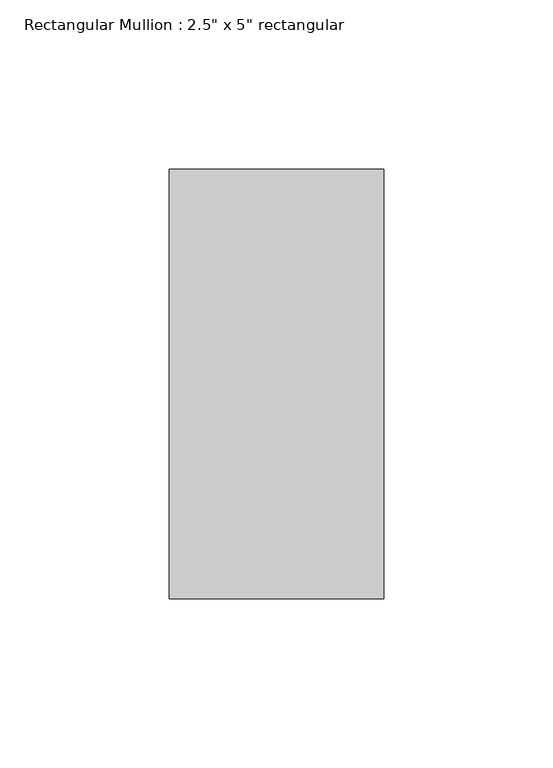
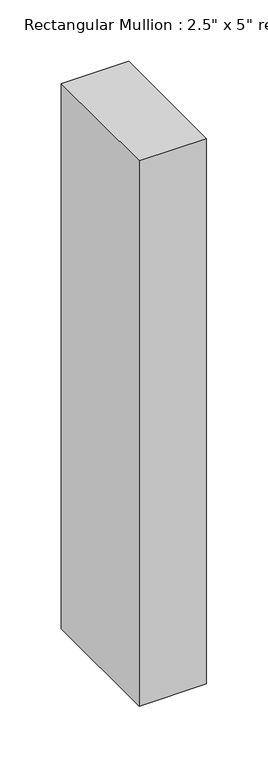
"""IFC4 building model written with IfcOpenShell, lengths in millimetres: member geometry."""

from ifc_helpers import new_model, si_unit, frame, origin, place, context, project, spatial, polyline, outline, extrude, source, transform, mapped, element, save


def member_255fa45d(model_context):
    return source(origin(), model_context, "Body", "SweptSolid", [
        extrude(outline(polyline([(31.75, 63.5), (31.75, -63.5), (-31.75, -63.5), (-31.75, 63.5), (31.75, 63.5)])), frame((0.0, 0.0, -544.1386718), z_axis=(0.0, 0.0, 1.0), x_axis=(1.0, 0.0, 0.0)), (0.0, 0.0, 1.0), 544.1386718),
    ])


if __name__ == "__main__":
    model = new_model("IFC4")
    model_context = context("Model", 3, world=origin())
    ifc_project = project(units=[si_unit("LENGTHUNIT", "METRE", prefix="MILLI")], contexts=[model_context])
    site = spatial("IfcSite", under=ifc_project)
    building = spatial("IfcBuilding", under=site)
    placement = place(None, origin())
    member_shape = member_255fa45d(model_context)
    element("IfcMember", 1, ObjectType="Rectangular Mullion : 2.5\" x 5\" rectangular", at=placement, inside=building, context=model_context, shape_type="MappedRepresentation", body=[
        mapped(member_shape, transform((0.0, 0.0, 0.0), x_axis=(1.0, 0.0, 0.0), y_axis=(0.0, 1.0, 0.0), z_axis=(0.0, 0.0, 1.0))),
    ])
    save(model, "model.ifc")

# Revit data of these elements
# Type "Rectangular Mullion : 2.5\" x 5\" rectangular"
#   built-in parameter 1007304 = 0.416667 (stored number, unit not read)
#   built-in parameter 1007301 = 0.104167 (stored number, unit not read)
#   built-in parameter 1007300 = 0.104167 (stored number, unit not read)
# Element 1 (IfcMember, "Rectangular Mullion : 2.5\" x 5\" rectangular")
#   Materials on its faces: "Aluminum"
# Materials
#   "Aluminum": class "Metal", colour RGB 247 247 247, transparency 0, Description = "Aluminum 6061", Cost = 0
